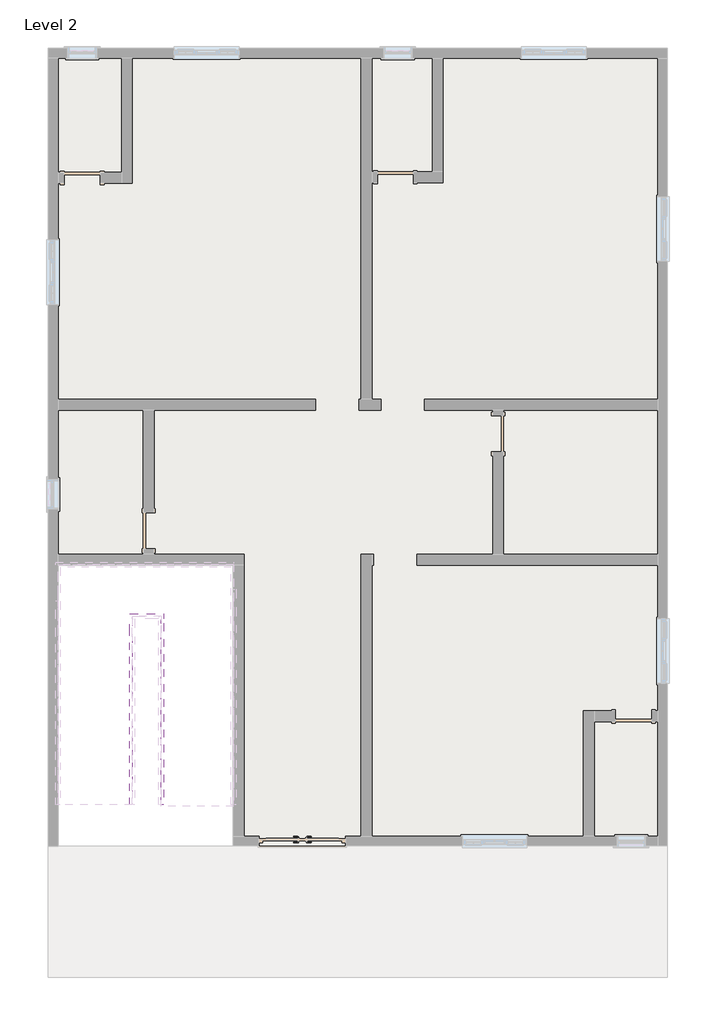
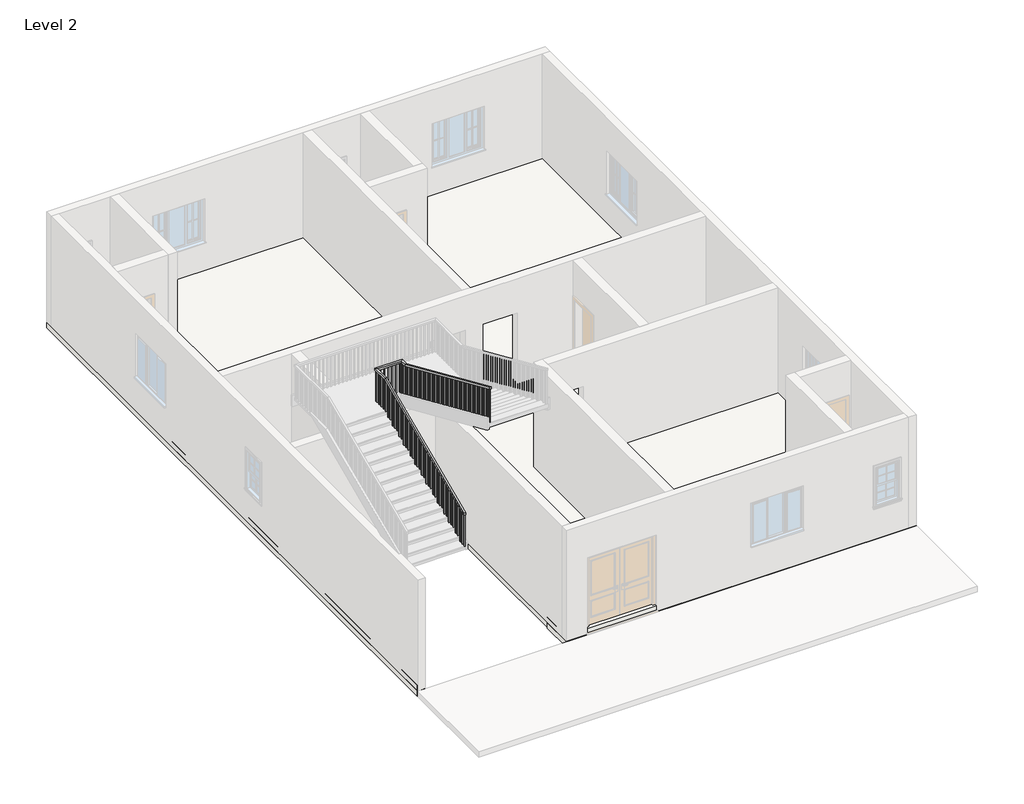
# One storey, part 2 of 4: 1 railing, 1 roof, 1 slab.
"""IFC4 building model written with IfcOpenShell, lengths in millimetres."""

from ifc_helpers import new_model, si_unit, frame, origin, place, context, project, spatial, polyline, outline, extrude, faceted_brep, element, save

model = new_model("IFC4")

# Units and contexts
model_context = context("Model", 3, world=origin())
ifc_project = project(units=[si_unit("LENGTHUNIT", "METRE", prefix="MILLI")], contexts=[model_context])

# Site, building, storey
site = spatial("IfcSite", under=ifc_project)
building = spatial("IfcBuilding", under=site)
storey = spatial("IfcBuildingStorey", under=building, Name="Level 2", Elevation=3048.0)

# Railing
placement = place(None, origin())
element("IfcRailing", 1, ObjectType="Handrail - Rectangular", at=placement, inside=storey, context=model_context, shape_type="SolidModel", body=[
    faceted_brep([(-6050.7290366, -6973.0610642, 6817.36), (-6050.7290366, -6973.0610642, 6761.8599828), (-5999.9290366, -6973.0610642, 6761.8599828), (-5999.9290366, -6973.0610642, 6817.36), (-6050.7290366, -3417.0610642, 8382.0), (-6050.7290366, -3406.3792071, 8331.2), (-5999.9290366, -3406.3792071, 8331.2), (-5999.9290366, -3417.0610642, 8382.0), (-6050.7290366, -2959.8610642, 8382.0), (-6050.7290366, -2959.8610642, 8331.2), (-5999.9290366, -3010.6610642, 8331.2), (-5999.9290366, -3010.6610642, 8382.0), (-5339.5290366, -2959.8610642, 8382.0), (-5339.5290366, -2959.8610642, 8331.2), (-5390.3290366, -3010.6610642, 8331.2), (-5390.3290366, -3010.6610642, 8382.0), (-5339.5290366, -3163.0610642, 8382.0), (-5339.5290366, -3173.7429214, 8331.2), (-5390.3290366, -3173.7429214, 8331.2), (-5390.3290366, -3163.0610642, 8382.0), (-5339.5290366, -6973.0610642, 10058.4), (-5390.3290366, -6973.0610642, 10058.4), (-5390.3290366, -6973.0610642, 10002.8999828), (-5339.5290366, -6973.0610642, 10002.8999828)], [[[0, 1, 2, 3]], [[1, 0, 4, 5]], [[2, 1, 5, 6]], [[3, 2, 6, 7]], [[0, 3, 7, 4]], [[5, 4, 8, 9]], [[6, 5, 9, 10]], [[7, 6, 10, 11]], [[4, 7, 11, 8]], [[9, 8, 12, 13]], [[10, 9, 13, 14]], [[11, 10, 14, 15]], [[8, 11, 15, 12]], [[13, 12, 16, 17]], [[14, 13, 17, 18]], [[15, 14, 18, 19]], [[12, 15, 19, 16]], [[20, 21, 22, 23]], [[17, 16, 20, 23]], [[18, 17, 23, 22]], [[19, 18, 22, 21]], [[16, 19, 21, 20]]]),
    extrude(outline(polyline([(-6957.1860642, 9995.9149828), (-6938.1360642, 9987.5329828), (-6938.1360642, 9032.24), (-6957.1860642, 9032.24), (-6957.1860642, 9995.9149828)])), frame((-5374.4540366, 0.0, 0.0), z_axis=(1.0, 0.0, 0.0), x_axis=(0.0, 1.0, 0.0)), (0.0, 0.0, 1.0), 19.05),
    extrude(outline(polyline([(-6855.5860642, 9951.2109828), (-6836.5360642, 9942.8289828), (-6836.5360642, 9032.24), (-6855.5860642, 9032.24), (-6855.5860642, 9951.2109828)])), frame((-5374.4540366, 0.0, 0.0), z_axis=(1.0, 0.0, 0.0), x_axis=(0.0, 1.0, 0.0)), (0.0, 0.0, 1.0), 19.05),
    extrude(outline(polyline([(-6753.9860642, 9906.5069828), (-6734.9360642, 9898.1249828), (-6734.9360642, 9032.24), (-6753.9860642, 9032.24), (-6753.9860642, 9906.5069828)])), frame((-5374.4540366, 0.0, 0.0), z_axis=(1.0, 0.0, 0.0), x_axis=(0.0, 1.0, 0.0)), (0.0, 0.0, 1.0), 19.05),
    extrude(outline(polyline([(-6652.3860642, 9861.8029828), (-6633.3360642, 9853.4209828), (-6633.3360642, 8920.48), (-6652.3860642, 8920.48), (-6652.3860642, 9861.8029828)])), frame((-5374.4540366, 0.0, 0.0), z_axis=(1.0, 0.0, 0.0), x_axis=(0.0, 1.0, 0.0)), (0.0, 0.0, 1.0), 19.05),
    extrude(outline(polyline([(-6550.7860642, 9817.0989828), (-6531.7360642, 9808.7169828), (-6531.7360642, 8920.48), (-6550.7860642, 8920.48), (-6550.7860642, 9817.0989828)])), frame((-5374.4540366, 0.0, 0.0), z_axis=(1.0, 0.0, 0.0), x_axis=(0.0, 1.0, 0.0)), (0.0, 0.0, 1.0), 19.05),
    extrude(outline(polyline([(-6449.1860642, 9772.3949828), (-6430.1360642, 9764.0129828), (-6430.1360642, 8808.72), (-6449.1860642, 8808.72), (-6449.1860642, 9772.3949828)])), frame((-5374.4540366, 0.0, 0.0), z_axis=(1.0, 0.0, 0.0), x_axis=(0.0, 1.0, 0.0)), (0.0, 0.0, 1.0), 19.05),
    extrude(outline(polyline([(-6347.5860642, 9727.6909828), (-6328.5360642, 9719.3089828), (-6328.5360642, 8808.72), (-6347.5860642, 8808.72), (-6347.5860642, 9727.6909828)])), frame((-5374.4540366, 0.0, 0.0), z_axis=(1.0, 0.0, 0.0), x_axis=(0.0, 1.0, 0.0)), (0.0, 0.0, 1.0), 19.05),
    extrude(outline(polyline([(-6245.9860642, 9682.9869828), (-6226.9360642, 9674.6049828), (-6226.9360642, 8808.72), (-6245.9860642, 8808.72), (-6245.9860642, 9682.9869828)])), frame((-5374.4540366, 0.0, 0.0), z_axis=(1.0, 0.0, 0.0), x_axis=(0.0, 1.0, 0.0)), (0.0, 0.0, 1.0), 19.05),
    extrude(outline(polyline([(-6144.3860642, 9638.2829828), (-6125.3360642, 9629.9009828), (-6125.3360642, 8696.96), (-6144.3860642, 8696.96), (-6144.3860642, 9638.2829828)])), frame((-5374.4540366, 0.0, 0.0), z_axis=(1.0, 0.0, 0.0), x_axis=(0.0, 1.0, 0.0)), (0.0, 0.0, 1.0), 19.05),
    extrude(outline(polyline([(-6042.7860642, 9593.5789828), (-6023.7360642, 9585.1969828), (-6023.7360642, 8696.96), (-6042.7860642, 8696.96), (-6042.7860642, 9593.5789828)])), frame((-5374.4540366, 0.0, 0.0), z_axis=(1.0, 0.0, 0.0), x_axis=(0.0, 1.0, 0.0)), (0.0, 0.0, 1.0), 19.05),
    extrude(outline(polyline([(-5941.1860642, 9548.8749828), (-5922.1360642, 9540.4929828), (-5922.1360642, 8585.2), (-5941.1860642, 8585.2), (-5941.1860642, 9548.8749828)])), frame((-5374.4540366, 0.0, 0.0), z_axis=(1.0, 0.0, 0.0), x_axis=(0.0, 1.0, 0.0)), (0.0, 0.0, 1.0), 19.05),
    extrude(outline(polyline([(-5839.5860642, 9504.1709828), (-5820.5360642, 9495.7889828), (-5820.5360642, 8585.2), (-5839.5860642, 8585.2), (-5839.5860642, 9504.1709828)])), frame((-5374.4540366, 0.0, 0.0), z_axis=(1.0, 0.0, 0.0), x_axis=(0.0, 1.0, 0.0)), (0.0, 0.0, 1.0), 19.05),
    extrude(outline(polyline([(-5737.9860642, 9459.4669828), (-5718.9360642, 9451.0849828), (-5718.9360642, 8585.2), (-5737.9860642, 8585.2), (-5737.9860642, 9459.4669828)])), frame((-5374.4540366, 0.0, 0.0), z_axis=(1.0, 0.0, 0.0), x_axis=(0.0, 1.0, 0.0)), (0.0, 0.0, 1.0), 19.05),
    extrude(outline(polyline([(-5636.3860642, 9414.7629828), (-5617.3360642, 9406.3809828), (-5617.3360642, 8473.44), (-5636.3860642, 8473.44), (-5636.3860642, 9414.7629828)])), frame((-5374.4540366, 0.0, 0.0), z_axis=(1.0, 0.0, 0.0), x_axis=(0.0, 1.0, 0.0)), (0.0, 0.0, 1.0), 19.05),
    extrude(outline(polyline([(-5534.7860642, 9370.0589828), (-5515.7360642, 9361.6769828), (-5515.7360642, 8473.44), (-5534.7860642, 8473.44), (-5534.7860642, 9370.0589828)])), frame((-5374.4540366, 0.0, 0.0), z_axis=(1.0, 0.0, 0.0), x_axis=(0.0, 1.0, 0.0)), (0.0, 0.0, 1.0), 19.05),
    extrude(outline(polyline([(-5433.1860642, 9325.3549828), (-5414.1360642, 9316.9729828), (-5414.1360642, 8361.68), (-5433.1860642, 8361.68), (-5433.1860642, 9325.3549828)])), frame((-5374.4540366, 0.0, 0.0), z_axis=(1.0, 0.0, 0.0), x_axis=(0.0, 1.0, 0.0)), (0.0, 0.0, 1.0), 19.05),
    extrude(outline(polyline([(-5331.5860642, 9280.6509828), (-5312.5360642, 9272.2689828), (-5312.5360642, 8361.68), (-5331.5860642, 8361.68), (-5331.5860642, 9280.6509828)])), frame((-5374.4540366, 0.0, 0.0), z_axis=(1.0, 0.0, 0.0), x_axis=(0.0, 1.0, 0.0)), (0.0, 0.0, 1.0), 19.05),
    extrude(outline(polyline([(-5229.9860642, 9235.9469828), (-5210.9360642, 9227.5649828), (-5210.9360642, 8361.68), (-5229.9860642, 8361.68), (-5229.9860642, 9235.9469828)])), frame((-5374.4540366, 0.0, 0.0), z_axis=(1.0, 0.0, 0.0), x_axis=(0.0, 1.0, 0.0)), (0.0, 0.0, 1.0), 19.05),
    extrude(outline(polyline([(-5128.3860642, 9191.2429828), (-5109.3360642, 9182.8609828), (-5109.3360642, 8249.92), (-5128.3860642, 8249.92), (-5128.3860642, 9191.2429828)])), frame((-5374.4540366, 0.0, 0.0), z_axis=(1.0, 0.0, 0.0), x_axis=(0.0, 1.0, 0.0)), (0.0, 0.0, 1.0), 19.05),
    extrude(outline(polyline([(-5026.7860642, 9146.5389828), (-5007.7360642, 9138.1569828), (-5007.7360642, 8249.92), (-5026.7860642, 8249.92), (-5026.7860642, 9146.5389828)])), frame((-5374.4540366, 0.0, 0.0), z_axis=(1.0, 0.0, 0.0), x_axis=(0.0, 1.0, 0.0)), (0.0, 0.0, 1.0), 19.05),
    extrude(outline(polyline([(-4925.1860642, 9101.8349828), (-4906.1360642, 9093.4529828), (-4906.1360642, 8138.16), (-4925.1860642, 8138.16), (-4925.1860642, 9101.8349828)])), frame((-5374.4540366, 0.0, 0.0), z_axis=(1.0, 0.0, 0.0), x_axis=(0.0, 1.0, 0.0)), (0.0, 0.0, 1.0), 19.05),
    extrude(outline(polyline([(-4823.5860642, 9057.1309828), (-4804.5360642, 9048.7489828), (-4804.5360642, 8138.16), (-4823.5860642, 8138.16), (-4823.5860642, 9057.1309828)])), frame((-5374.4540366, 0.0, 0.0), z_axis=(1.0, 0.0, 0.0), x_axis=(0.0, 1.0, 0.0)), (0.0, 0.0, 1.0), 19.05),
    extrude(outline(polyline([(-4721.9860642, 9012.4269828), (-4702.9360642, 9004.0449828), (-4702.9360642, 8138.16), (-4721.9860642, 8138.16), (-4721.9860642, 9012.4269828)])), frame((-5374.4540366, 0.0, 0.0), z_axis=(1.0, 0.0, 0.0), x_axis=(0.0, 1.0, 0.0)), (0.0, 0.0, 1.0), 19.05),
    extrude(outline(polyline([(-4620.3860642, 8967.7229828), (-4601.3360642, 8959.3409828), (-4601.3360642, 8026.4), (-4620.3860642, 8026.4), (-4620.3860642, 8967.7229828)])), frame((-5374.4540366, 0.0, 0.0), z_axis=(1.0, 0.0, 0.0), x_axis=(0.0, 1.0, 0.0)), (0.0, 0.0, 1.0), 19.05),
    extrude(outline(polyline([(-4518.7860642, 8923.0189828), (-4499.7360642, 8914.6369828), (-4499.7360642, 8026.4), (-4518.7860642, 8026.4), (-4518.7860642, 8923.0189828)])), frame((-5374.4540366, 0.0, 0.0), z_axis=(1.0, 0.0, 0.0), x_axis=(0.0, 1.0, 0.0)), (0.0, 0.0, 1.0), 19.05),
    extrude(outline(polyline([(-4417.1860642, 8878.3149828), (-4398.1360642, 8869.9329828), (-4398.1360642, 7914.64), (-4417.1860642, 7914.64), (-4417.1860642, 8878.3149828)])), frame((-5374.4540366, 0.0, 0.0), z_axis=(1.0, 0.0, 0.0), x_axis=(0.0, 1.0, 0.0)), (0.0, 0.0, 1.0), 19.05),
    extrude(outline(polyline([(-4315.5860642, 8833.6109828), (-4296.5360642, 8825.2289828), (-4296.5360642, 7914.64), (-4315.5860642, 7914.64), (-4315.5860642, 8833.6109828)])), frame((-5374.4540366, 0.0, 0.0), z_axis=(1.0, 0.0, 0.0), x_axis=(0.0, 1.0, 0.0)), (0.0, 0.0, 1.0), 19.05),
    extrude(outline(polyline([(-4213.9860642, 8788.9069828), (-4194.9360642, 8780.5249828), (-4194.9360642, 7914.64), (-4213.9860642, 7914.64), (-4213.9860642, 8788.9069828)])), frame((-5374.4540366, 0.0, 0.0), z_axis=(1.0, 0.0, 0.0), x_axis=(0.0, 1.0, 0.0)), (0.0, 0.0, 1.0), 19.05),
    extrude(outline(polyline([(-4112.3860642, 8744.2029828), (-4093.3360642, 8735.8209828), (-4093.3360642, 7802.88), (-4112.3860642, 7802.88), (-4112.3860642, 8744.2029828)])), frame((-5374.4540366, 0.0, 0.0), z_axis=(1.0, 0.0, 0.0), x_axis=(0.0, 1.0, 0.0)), (0.0, 0.0, 1.0), 19.05),
    extrude(outline(polyline([(-4010.7860642, 8699.4989828), (-3991.7360642, 8691.1169828), (-3991.7360642, 7802.88), (-4010.7860642, 7802.88), (-4010.7860642, 8699.4989828)])), frame((-5374.4540366, 0.0, 0.0), z_axis=(1.0, 0.0, 0.0), x_axis=(0.0, 1.0, 0.0)), (0.0, 0.0, 1.0), 19.05),
    extrude(outline(polyline([(-3909.1860642, 8654.7949828), (-3890.1360642, 8646.4129828), (-3890.1360642, 7691.12), (-3909.1860642, 7691.12), (-3909.1860642, 8654.7949828)])), frame((-5374.4540366, 0.0, 0.0), z_axis=(1.0, 0.0, 0.0), x_axis=(0.0, 1.0, 0.0)), (0.0, 0.0, 1.0), 19.05),
    extrude(outline(polyline([(-3807.5860642, 8610.0909828), (-3788.5360642, 8601.7089828), (-3788.5360642, 7691.12), (-3807.5860642, 7691.12), (-3807.5860642, 8610.0909828)])), frame((-5374.4540366, 0.0, 0.0), z_axis=(1.0, 0.0, 0.0), x_axis=(0.0, 1.0, 0.0)), (0.0, 0.0, 1.0), 19.05),
    extrude(outline(polyline([(-3705.9860642, 8565.3869828), (-3686.9360642, 8557.0049828), (-3686.9360642, 7691.12), (-3705.9860642, 7691.12), (-3705.9860642, 8565.3869828)])), frame((-5374.4540366, 0.0, 0.0), z_axis=(1.0, 0.0, 0.0), x_axis=(0.0, 1.0, 0.0)), (0.0, 0.0, 1.0), 19.05),
    extrude(outline(polyline([(-3604.3860642, 8520.6829828), (-3585.3360642, 8512.3009828), (-3585.3360642, 7579.36), (-3604.3860642, 7579.36), (-3604.3860642, 8520.6829828)])), frame((-5374.4540366, 0.0, 0.0), z_axis=(1.0, 0.0, 0.0), x_axis=(0.0, 1.0, 0.0)), (0.0, 0.0, 1.0), 19.05),
    extrude(outline(polyline([(-3502.7860642, 8475.9789828), (-3483.7360642, 8467.5969828), (-3483.7360642, 7579.36), (-3502.7860642, 7579.36), (-3502.7860642, 8475.9789828)])), frame((-5374.4540366, 0.0, 0.0), z_axis=(1.0, 0.0, 0.0), x_axis=(0.0, 1.0, 0.0)), (0.0, 0.0, 1.0), 19.05),
    extrude(outline(polyline([(-3401.1860642, 8431.2749828), (-3382.1360642, 8422.8929828), (-3382.1360642, 7467.6), (-3401.1860642, 7467.6), (-3401.1860642, 8431.2749828)])), frame((-5374.4540366, 0.0, 0.0), z_axis=(1.0, 0.0, 0.0), x_axis=(0.0, 1.0, 0.0)), (0.0, 0.0, 1.0), 19.05),
    extrude(outline(polyline([(-3299.5860642, 8386.5709828), (-3280.5360642, 8378.1889828), (-3280.5360642, 7467.6), (-3299.5860642, 7467.6), (-3299.5860642, 8386.5709828)])), frame((-5374.4540366, 0.0, 0.0), z_axis=(1.0, 0.0, 0.0), x_axis=(0.0, 1.0, 0.0)), (0.0, 0.0, 1.0), 19.05),
    extrude(outline(polyline([(-3197.9860642, 8341.8669828), (-3178.9360642, 8333.4849828), (-3178.9360642, 7467.6), (-3197.9860642, 7467.6), (-3197.9860642, 8341.8669828)])), frame((-5374.4540366, 0.0, 0.0), z_axis=(1.0, 0.0, 0.0), x_axis=(0.0, 1.0, 0.0)), (0.0, 0.0, 1.0), 19.05),
    extrude(outline(polyline([(-5374.4540366, -3077.3360642), (-5355.4040366, -3077.3360642), (-5355.4040366, -3096.3860642), (-5374.4540366, -3096.3860642), (-5374.4540366, -3077.3360642)])), frame((0.0, 0.0, 7467.6), z_axis=(0.0, 0.0, 1.0), x_axis=(1.0, 0.0, 0.0)), (0.0, 0.0, 1.0), 863.6),
    extrude(outline(polyline([(-5425.2540366, -2994.7860642), (-5425.2540366, -2975.7360642), (-5406.2040366, -2975.7360642), (-5406.2040366, -2994.7860642), (-5425.2540366, -2994.7860642)])), frame((0.0, 0.0, 7467.6), z_axis=(0.0, 0.0, 1.0), x_axis=(1.0, 0.0, 0.0)), (0.0, 0.0, 1.0), 863.6),
    extrude(outline(polyline([(-5526.8540366, -2994.7860642), (-5526.8540366, -2975.7360642), (-5507.8040366, -2975.7360642), (-5507.8040366, -2994.7860642), (-5526.8540366, -2994.7860642)])), frame((0.0, 0.0, 7467.6), z_axis=(0.0, 0.0, 1.0), x_axis=(1.0, 0.0, 0.0)), (0.0, 0.0, 1.0), 863.6),
    extrude(outline(polyline([(-5628.4540366, -2994.7860642), (-5628.4540366, -2975.7360642), (-5609.4040366, -2975.7360642), (-5609.4040366, -2994.7860642), (-5628.4540366, -2994.7860642)])), frame((0.0, 0.0, 7467.6), z_axis=(0.0, 0.0, 1.0), x_axis=(1.0, 0.0, 0.0)), (0.0, 0.0, 1.0), 863.6),
    extrude(outline(polyline([(-5730.0540366, -2994.7860642), (-5730.0540366, -2975.7360642), (-5711.0040366, -2975.7360642), (-5711.0040366, -2994.7860642), (-5730.0540366, -2994.7860642)])), frame((0.0, 0.0, 7467.6), z_axis=(0.0, 0.0, 1.0), x_axis=(1.0, 0.0, 0.0)), (0.0, 0.0, 1.0), 863.6),
    extrude(outline(polyline([(-5831.6540366, -2994.7860642), (-5831.6540366, -2975.7360642), (-5812.6040366, -2975.7360642), (-5812.6040366, -2994.7860642), (-5831.6540366, -2994.7860642)])), frame((0.0, 0.0, 7467.6), z_axis=(0.0, 0.0, 1.0), x_axis=(1.0, 0.0, 0.0)), (0.0, 0.0, 1.0), 863.6),
    extrude(outline(polyline([(-5933.2540366, -2994.7860642), (-5933.2540366, -2975.7360642), (-5914.2040366, -2975.7360642), (-5914.2040366, -2994.7860642), (-5933.2540366, -2994.7860642)])), frame((0.0, 0.0, 7467.6), z_axis=(0.0, 0.0, 1.0), x_axis=(1.0, 0.0, 0.0)), (0.0, 0.0, 1.0), 863.6),
    extrude(outline(polyline([(-6015.8040366, -3020.1860642), (-6034.8540366, -3020.1860642), (-6034.8540366, -3001.1360642), (-6015.8040366, -3001.1360642), (-6015.8040366, -3020.1860642)])), frame((0.0, 0.0, 7467.6), z_axis=(0.0, 0.0, 1.0), x_axis=(1.0, 0.0, 0.0)), (0.0, 0.0, 1.0), 863.6),
    extrude(outline(polyline([(-6015.8040366, -3121.7860642), (-6034.8540366, -3121.7860642), (-6034.8540366, -3102.7360642), (-6015.8040366, -3102.7360642), (-6015.8040366, -3121.7860642)])), frame((0.0, 0.0, 7467.6), z_axis=(0.0, 0.0, 1.0), x_axis=(1.0, 0.0, 0.0)), (0.0, 0.0, 1.0), 863.6),
    extrude(outline(polyline([(-6015.8040366, -3223.3860642), (-6034.8540366, -3223.3860642), (-6034.8540366, -3204.3360642), (-6015.8040366, -3204.3360642), (-6015.8040366, -3223.3860642)])), frame((0.0, 0.0, 7467.6), z_axis=(0.0, 0.0, 1.0), x_axis=(1.0, 0.0, 0.0)), (0.0, 0.0, 1.0), 863.6),
    extrude(outline(polyline([(-6015.8040366, -3324.9860642), (-6034.8540366, -3324.9860642), (-6034.8540366, -3305.9360642), (-6015.8040366, -3305.9360642), (-6015.8040366, -3324.9860642)])), frame((0.0, 0.0, 7467.6), z_axis=(0.0, 0.0, 1.0), x_axis=(1.0, 0.0, 0.0)), (0.0, 0.0, 1.0), 863.6),
    extrude(outline(polyline([(-3426.5860642, 8322.3089828), (-3407.5360642, 8330.6909828), (-3407.5360642, 7467.6), (-3426.5860642, 7467.6), (-3426.5860642, 8322.3089828)])), frame((-6034.8540366, 0.0, 0.0), z_axis=(1.0, 0.0, 0.0), x_axis=(0.0, 1.0, 0.0)), (0.0, 0.0, 1.0), 19.05),
    extrude(outline(polyline([(-3528.1860642, 8277.6049828), (-3509.1360642, 8285.9869828), (-3509.1360642, 7355.84), (-3528.1860642, 7355.84), (-3528.1860642, 8277.6049828)])), frame((-6034.8540366, 0.0, 0.0), z_axis=(1.0, 0.0, 0.0), x_axis=(0.0, 1.0, 0.0)), (0.0, 0.0, 1.0), 19.05),
    extrude(outline(polyline([(-3629.7860642, 8232.9009828), (-3610.7360642, 8241.2829828), (-3610.7360642, 7355.84), (-3629.7860642, 7355.84), (-3629.7860642, 8232.9009828)])), frame((-6034.8540366, 0.0, 0.0), z_axis=(1.0, 0.0, 0.0), x_axis=(0.0, 1.0, 0.0)), (0.0, 0.0, 1.0), 19.05),
    extrude(outline(polyline([(-3731.3860642, 8188.1969828), (-3712.3360642, 8196.5789828), (-3712.3360642, 7244.08), (-3731.3860642, 7244.08), (-3731.3860642, 8188.1969828)])), frame((-6034.8540366, 0.0, 0.0), z_axis=(1.0, 0.0, 0.0), x_axis=(0.0, 1.0, 0.0)), (0.0, 0.0, 1.0), 19.05),
    extrude(outline(polyline([(-3832.9860642, 8143.4929828), (-3813.9360642, 8151.8749828), (-3813.9360642, 7244.08), (-3832.9860642, 7244.08), (-3832.9860642, 8143.4929828)])), frame((-6034.8540366, 0.0, 0.0), z_axis=(1.0, 0.0, 0.0), x_axis=(0.0, 1.0, 0.0)), (0.0, 0.0, 1.0), 19.05),
    extrude(outline(polyline([(-3934.5860642, 8098.7889828), (-3915.5360642, 8107.1709828), (-3915.5360642, 7244.08), (-3934.5860642, 7244.08), (-3934.5860642, 8098.7889828)])), frame((-6034.8540366, 0.0, 0.0), z_axis=(1.0, 0.0, 0.0), x_axis=(0.0, 1.0, 0.0)), (0.0, 0.0, 1.0), 19.05),
    extrude(outline(polyline([(-4036.1860642, 8054.0849828), (-4017.1360642, 8062.4669828), (-4017.1360642, 7132.32), (-4036.1860642, 7132.32), (-4036.1860642, 8054.0849828)])), frame((-6034.8540366, 0.0, 0.0), z_axis=(1.0, 0.0, 0.0), x_axis=(0.0, 1.0, 0.0)), (0.0, 0.0, 1.0), 19.05),
    extrude(outline(polyline([(-4137.7860642, 8009.3809828), (-4118.7360642, 8017.7629828), (-4118.7360642, 7132.32), (-4137.7860642, 7132.32), (-4137.7860642, 8009.3809828)])), frame((-6034.8540366, 0.0, 0.0), z_axis=(1.0, 0.0, 0.0), x_axis=(0.0, 1.0, 0.0)), (0.0, 0.0, 1.0), 19.05),
    extrude(outline(polyline([(-4239.3860642, 7964.6769828), (-4220.3360642, 7973.0589828), (-4220.3360642, 7020.56), (-4239.3860642, 7020.56), (-4239.3860642, 7964.6769828)])), frame((-6034.8540366, 0.0, 0.0), z_axis=(1.0, 0.0, 0.0), x_axis=(0.0, 1.0, 0.0)), (0.0, 0.0, 1.0), 19.05),
    extrude(outline(polyline([(-4340.9860642, 7919.9729828), (-4321.9360642, 7928.3549828), (-4321.9360642, 7020.56), (-4340.9860642, 7020.56), (-4340.9860642, 7919.9729828)])), frame((-6034.8540366, 0.0, 0.0), z_axis=(1.0, 0.0, 0.0), x_axis=(0.0, 1.0, 0.0)), (0.0, 0.0, 1.0), 19.05),
    extrude(outline(polyline([(-4442.5860642, 7875.2689828), (-4423.5360642, 7883.6509828), (-4423.5360642, 7020.56), (-4442.5860642, 7020.56), (-4442.5860642, 7875.2689828)])), frame((-6034.8540366, 0.0, 0.0), z_axis=(1.0, 0.0, 0.0), x_axis=(0.0, 1.0, 0.0)), (0.0, 0.0, 1.0), 19.05),
    extrude(outline(polyline([(-4544.1860642, 7830.5649828), (-4525.1360642, 7838.9469828), (-4525.1360642, 6908.8), (-4544.1860642, 6908.8), (-4544.1860642, 7830.5649828)])), frame((-6034.8540366, 0.0, 0.0), z_axis=(1.0, 0.0, 0.0), x_axis=(0.0, 1.0, 0.0)), (0.0, 0.0, 1.0), 19.05),
    extrude(outline(polyline([(-4645.7860642, 7785.8609828), (-4626.7360642, 7794.2429828), (-4626.7360642, 6908.8), (-4645.7860642, 6908.8), (-4645.7860642, 7785.8609828)])), frame((-6034.8540366, 0.0, 0.0), z_axis=(1.0, 0.0, 0.0), x_axis=(0.0, 1.0, 0.0)), (0.0, 0.0, 1.0), 19.05),
    extrude(outline(polyline([(-4747.3860642, 7741.1569828), (-4728.3360642, 7749.5389828), (-4728.3360642, 6797.04), (-4747.3860642, 6797.04), (-4747.3860642, 7741.1569828)])), frame((-6034.8540366, 0.0, 0.0), z_axis=(1.0, 0.0, 0.0), x_axis=(0.0, 1.0, 0.0)), (0.0, 0.0, 1.0), 19.05),
    extrude(outline(polyline([(-4848.9860642, 7696.4529828), (-4829.9360642, 7704.8349828), (-4829.9360642, 6797.04), (-4848.9860642, 6797.04), (-4848.9860642, 7696.4529828)])), frame((-6034.8540366, 0.0, 0.0), z_axis=(1.0, 0.0, 0.0), x_axis=(0.0, 1.0, 0.0)), (0.0, 0.0, 1.0), 19.05),
    extrude(outline(polyline([(-4950.5860642, 7651.7489828), (-4931.5360642, 7660.1309828), (-4931.5360642, 6797.04), (-4950.5860642, 6797.04), (-4950.5860642, 7651.7489828)])), frame((-6034.8540366, 0.0, 0.0), z_axis=(1.0, 0.0, 0.0), x_axis=(0.0, 1.0, 0.0)), (0.0, 0.0, 1.0), 19.05),
    extrude(outline(polyline([(-5052.1860642, 7607.0449828), (-5033.1360642, 7615.4269828), (-5033.1360642, 6685.28), (-5052.1860642, 6685.28), (-5052.1860642, 7607.0449828)])), frame((-6034.8540366, 0.0, 0.0), z_axis=(1.0, 0.0, 0.0), x_axis=(0.0, 1.0, 0.0)), (0.0, 0.0, 1.0), 19.05),
    extrude(outline(polyline([(-5153.7860642, 7562.3409828), (-5134.7360642, 7570.7229828), (-5134.7360642, 6685.28), (-5153.7860642, 6685.28), (-5153.7860642, 7562.3409828)])), frame((-6034.8540366, 0.0, 0.0), z_axis=(1.0, 0.0, 0.0), x_axis=(0.0, 1.0, 0.0)), (0.0, 0.0, 1.0), 19.05),
    extrude(outline(polyline([(-5255.3860642, 7517.6369828), (-5236.3360642, 7526.0189828), (-5236.3360642, 6573.52), (-5255.3860642, 6573.52), (-5255.3860642, 7517.6369828)])), frame((-6034.8540366, 0.0, 0.0), z_axis=(1.0, 0.0, 0.0), x_axis=(0.0, 1.0, 0.0)), (0.0, 0.0, 1.0), 19.05),
    extrude(outline(polyline([(-5356.9860642, 7472.9329828), (-5337.9360642, 7481.3149828), (-5337.9360642, 6573.52), (-5356.9860642, 6573.52), (-5356.9860642, 7472.9329828)])), frame((-6034.8540366, 0.0, 0.0), z_axis=(1.0, 0.0, 0.0), x_axis=(0.0, 1.0, 0.0)), (0.0, 0.0, 1.0), 19.05),
    extrude(outline(polyline([(-5458.5860642, 7428.2289828), (-5439.5360642, 7436.6109828), (-5439.5360642, 6573.52), (-5458.5860642, 6573.52), (-5458.5860642, 7428.2289828)])), frame((-6034.8540366, 0.0, 0.0), z_axis=(1.0, 0.0, 0.0), x_axis=(0.0, 1.0, 0.0)), (0.0, 0.0, 1.0), 19.05),
    extrude(outline(polyline([(-5560.1860642, 7383.5249828), (-5541.1360642, 7391.9069828), (-5541.1360642, 6461.76), (-5560.1860642, 6461.76), (-5560.1860642, 7383.5249828)])), frame((-6034.8540366, 0.0, 0.0), z_axis=(1.0, 0.0, 0.0), x_axis=(0.0, 1.0, 0.0)), (0.0, 0.0, 1.0), 19.05),
    extrude(outline(polyline([(-5661.7860642, 7338.8209828), (-5642.7360642, 7347.2029828), (-5642.7360642, 6461.76), (-5661.7860642, 6461.76), (-5661.7860642, 7338.8209828)])), frame((-6034.8540366, 0.0, 0.0), z_axis=(1.0, 0.0, 0.0), x_axis=(0.0, 1.0, 0.0)), (0.0, 0.0, 1.0), 19.05),
    extrude(outline(polyline([(-5763.3860642, 7294.1169828), (-5744.3360642, 7302.4989828), (-5744.3360642, 6350.0), (-5763.3860642, 6350.0), (-5763.3860642, 7294.1169828)])), frame((-6034.8540366, 0.0, 0.0), z_axis=(1.0, 0.0, 0.0), x_axis=(0.0, 1.0, 0.0)), (0.0, 0.0, 1.0), 19.05),
    extrude(outline(polyline([(-5864.9860642, 7249.4129828), (-5845.9360642, 7257.7949828), (-5845.9360642, 6350.0), (-5864.9860642, 6350.0), (-5864.9860642, 7249.4129828)])), frame((-6034.8540366, 0.0, 0.0), z_axis=(1.0, 0.0, 0.0), x_axis=(0.0, 1.0, 0.0)), (0.0, 0.0, 1.0), 19.05),
    extrude(outline(polyline([(-5966.5860642, 7204.7089828), (-5947.5360642, 7213.0909828), (-5947.5360642, 6350.0), (-5966.5860642, 6350.0), (-5966.5860642, 7204.7089828)])), frame((-6034.8540366, 0.0, 0.0), z_axis=(1.0, 0.0, 0.0), x_axis=(0.0, 1.0, 0.0)), (0.0, 0.0, 1.0), 19.05),
    extrude(outline(polyline([(-6068.1860642, 7160.0049828), (-6049.1360642, 7168.3869828), (-6049.1360642, 6238.24), (-6068.1860642, 6238.24), (-6068.1860642, 7160.0049828)])), frame((-6034.8540366, 0.0, 0.0), z_axis=(1.0, 0.0, 0.0), x_axis=(0.0, 1.0, 0.0)), (0.0, 0.0, 1.0), 19.05),
    extrude(outline(polyline([(-6169.7860642, 7115.3009828), (-6150.7360642, 7123.6829828), (-6150.7360642, 6238.24), (-6169.7860642, 6238.24), (-6169.7860642, 7115.3009828)])), frame((-6034.8540366, 0.0, 0.0), z_axis=(1.0, 0.0, 0.0), x_axis=(0.0, 1.0, 0.0)), (0.0, 0.0, 1.0), 19.05),
    extrude(outline(polyline([(-6271.3860642, 7070.5969828), (-6252.3360642, 7078.9789828), (-6252.3360642, 6126.48), (-6271.3860642, 6126.48), (-6271.3860642, 7070.5969828)])), frame((-6034.8540366, 0.0, 0.0), z_axis=(1.0, 0.0, 0.0), x_axis=(0.0, 1.0, 0.0)), (0.0, 0.0, 1.0), 19.05),
    extrude(outline(polyline([(-6372.9860642, 7025.8929828), (-6353.9360642, 7034.2749828), (-6353.9360642, 6126.48), (-6372.9860642, 6126.48), (-6372.9860642, 7025.8929828)])), frame((-6034.8540366, 0.0, 0.0), z_axis=(1.0, 0.0, 0.0), x_axis=(0.0, 1.0, 0.0)), (0.0, 0.0, 1.0), 19.05),
    extrude(outline(polyline([(-6474.5860642, 6981.1889828), (-6455.5360642, 6989.5709828), (-6455.5360642, 6126.48), (-6474.5860642, 6126.48), (-6474.5860642, 6981.1889828)])), frame((-6034.8540366, 0.0, 0.0), z_axis=(1.0, 0.0, 0.0), x_axis=(0.0, 1.0, 0.0)), (0.0, 0.0, 1.0), 19.05),
    extrude(outline(polyline([(-6576.1860642, 6936.4849828), (-6557.1360642, 6944.8669828), (-6557.1360642, 6014.72), (-6576.1860642, 6014.72), (-6576.1860642, 6936.4849828)])), frame((-6034.8540366, 0.0, 0.0), z_axis=(1.0, 0.0, 0.0), x_axis=(0.0, 1.0, 0.0)), (0.0, 0.0, 1.0), 19.05),
    extrude(outline(polyline([(-6677.7860642, 6891.7809828), (-6658.7360642, 6900.1629828), (-6658.7360642, 6014.72), (-6677.7860642, 6014.72), (-6677.7860642, 6891.7809828)])), frame((-6034.8540366, 0.0, 0.0), z_axis=(1.0, 0.0, 0.0), x_axis=(0.0, 1.0, 0.0)), (0.0, 0.0, 1.0), 19.05),
    extrude(outline(polyline([(-6779.3860642, 6847.0769828), (-6760.3360642, 6855.4589828), (-6760.3360642, 5902.96), (-6779.3860642, 5902.96), (-6779.3860642, 6847.0769828)])), frame((-6034.8540366, 0.0, 0.0), z_axis=(1.0, 0.0, 0.0), x_axis=(0.0, 1.0, 0.0)), (0.0, 0.0, 1.0), 19.05),
    extrude(outline(polyline([(-6880.9860642, 6802.3729828), (-6861.9360642, 6810.7549828), (-6861.9360642, 5902.96), (-6880.9860642, 5902.96), (-6880.9860642, 6802.3729828)])), frame((-6034.8540366, 0.0, 0.0), z_axis=(1.0, 0.0, 0.0), x_axis=(0.0, 1.0, 0.0)), (0.0, 0.0, 1.0), 19.05),
    extrude(outline(polyline([(-5374.4540366, -2994.7860642), (-5374.4540366, -2975.7360642), (-5355.4040366, -2975.7360642), (-5355.4040366, -2994.7860642), (-5374.4540366, -2994.7860642)])), frame((0.0, 0.0, 7467.6), z_axis=(0.0, 0.0, 1.0), x_axis=(1.0, 0.0, 0.0)), (0.0, 0.0, 1.0), 863.6),
    extrude(outline(polyline([(-6015.8040366, -2994.7860642), (-6034.8540366, -2994.7860642), (-6034.8540366, -2975.7360642), (-6015.8040366, -2975.7360642), (-6015.8040366, -2994.7860642)])), frame((0.0, 0.0, 7467.6), z_axis=(0.0, 0.0, 1.0), x_axis=(1.0, 0.0, 0.0)), (0.0, 0.0, 1.0), 863.6),
    extrude(outline(polyline([(-6973.0610642, 10002.8999828), (-6954.0110642, 9994.5179828), (-6954.0110642, 9032.24), (-6973.0610642, 9032.24), (-6973.0610642, 10002.8999828)])), frame((-5374.4540366, 0.0, 0.0), z_axis=(1.0, 0.0, 0.0), x_axis=(0.0, 1.0, 0.0)), (0.0, 0.0, 1.0), 19.05),
    extrude(outline(polyline([(-6973.0610642, 6761.8599828), (-6954.0110642, 6770.2419828), (-6954.0110642, 5902.96), (-6973.0610642, 5902.96), (-6973.0610642, 6761.8599828)])), frame((-6034.8540366, 0.0, 0.0), z_axis=(1.0, 0.0, 0.0), x_axis=(0.0, 1.0, 0.0)), (0.0, 0.0, 1.0), 19.05),
])

# Roof
element("IfcRoof", 2, ObjectType="Generic - 12\"", at=placement, inside=storey, context=model_context, shape_type="SweptSolid", body=[
    extrude(outline(polyline([(-7757.6415084, 8907.4935985), (5247.1584916, 8907.4935985), (5247.1584916, -7831.1064015), (-3879.0290366, -7831.1064015), (-3879.0290366, -6973.0610642), (-3866.3290366, -6973.0610642), (-3866.3290366, -1928.4217109), (-7554.4415084, -1928.4217109), (-7554.4415084, -7831.1064015), (-7757.6415084, -7831.1064015), (-7757.6415084, 8907.4935985)])), frame((0.0, 0.0, 3048.0), z_axis=(0.0, 0.0, 1.0), x_axis=(1.0, 0.0, 0.0)), (0.0, 0.0, 1.0), 152.4),
])

# Slab
element("IfcSlab", 3, ObjectType="Generic - 12\"", at=placement, inside=storey, context=model_context, shape_type="SweptSolid", body=[
    extrude(outline(polyline([(5247.1584916, 8907.4935985), (5247.1584916, -7831.1064015), (-3879.0290366, -7831.1064015), (-3879.0290366, -6973.0610642), (-3866.3290366, -6973.0610642), (-3866.3290366, -1928.4217109), (-7554.4415084, -1928.4217109), (-7554.4415084, -7831.1064015), (-7757.6415084, -7831.1064015), (-7757.6415084, 8907.4935985), (5247.1584916, 8907.4935985)])), frame((0.0, 0.0, 2895.6), z_axis=(0.0, 0.0, 1.0), x_axis=(1.0, 0.0, 0.0)), (0.0, 0.0, 1.0), 152.4),
])

save(model, "model.ifc")

# Revit data of these elements
# Type "Handrail - Rectangular"
#   Assembly Code = "C2010400"
#   built-in parameter 1008612 = 0.0416667 (stored number, unit not read)
#   built-in parameter 1008611 = 0.0416667 (stored number, unit not read)
#   built-in parameter 1008609 = 0.333333 (stored number, unit not read)
#   built-in parameter 1008604 = 0.166667 (stored number, unit not read)
#   built-in parameter 1008603 = 0.166667 (stored number, unit not read)
#   Railing Height = 3' - 0"
#   built-in parameter 1008630 = 2
#   built-in parameter 1008610 = 2
#   built-in parameter 1008618 = Baluster - Square : 3/4"
# Type "Generic - 12\""
#   Assembly Code = "B1020"
#   Layers, outside or top first: 0' - 6" no material (function 1)
# Type "Generic - 12\""
#   Assembly Code = "B1010"
#   Function = 0
#   Layers, outside or top first: 0' - 6" no material (function 1)
# Element 1 (IfcRailing, "Handrail - Rectangular")
#   Phase Created = New Construction
# Element 2 (IfcRoof, "Generic - 12\"")
#   built-in parameter 1001705 = 10.5 (stored number, unit not read)
#   built-in parameter 1001710 = 33615
#   Phase Created = New Construction
#   Materials on its faces: "Default Roof"
# Element 3 (IfcSlab, "Generic - 12\"")
#   Height Offset From Level = 0' - 0"
#   Phase Created = New Construction
#   Materials on its faces: "Default Floor"
# Materials
#   "Default Roof": colour RGB 88 101 114, transparency 0, Cost = 0
#   "Default Floor": colour RGB 128 128 128, transparency 0, Cost = 0
